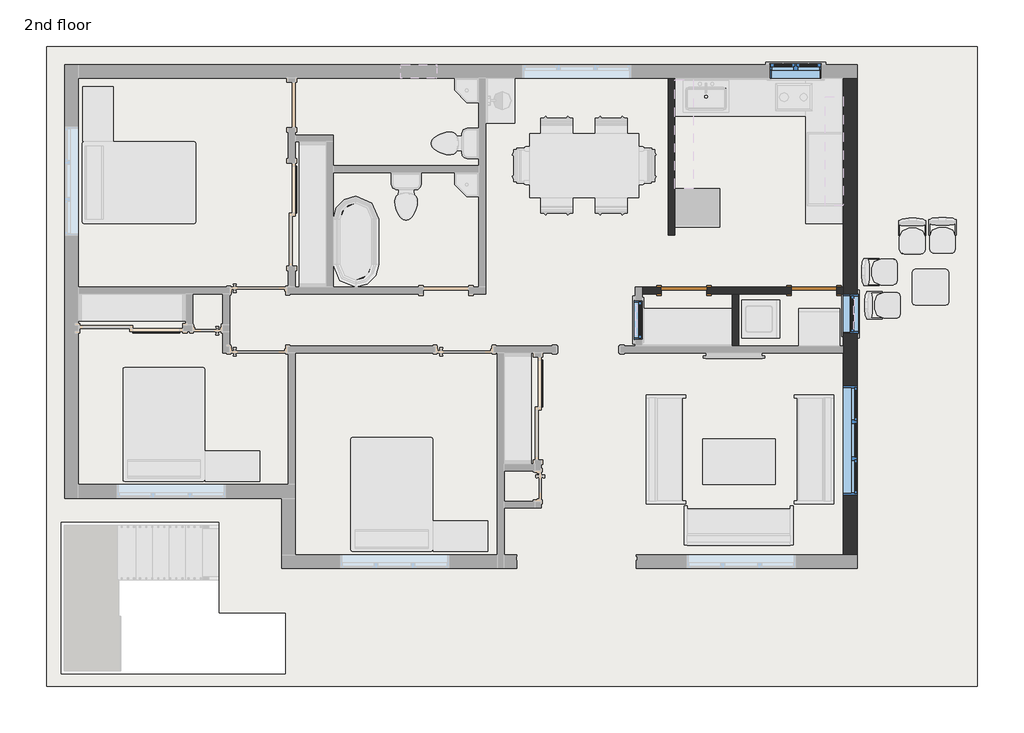
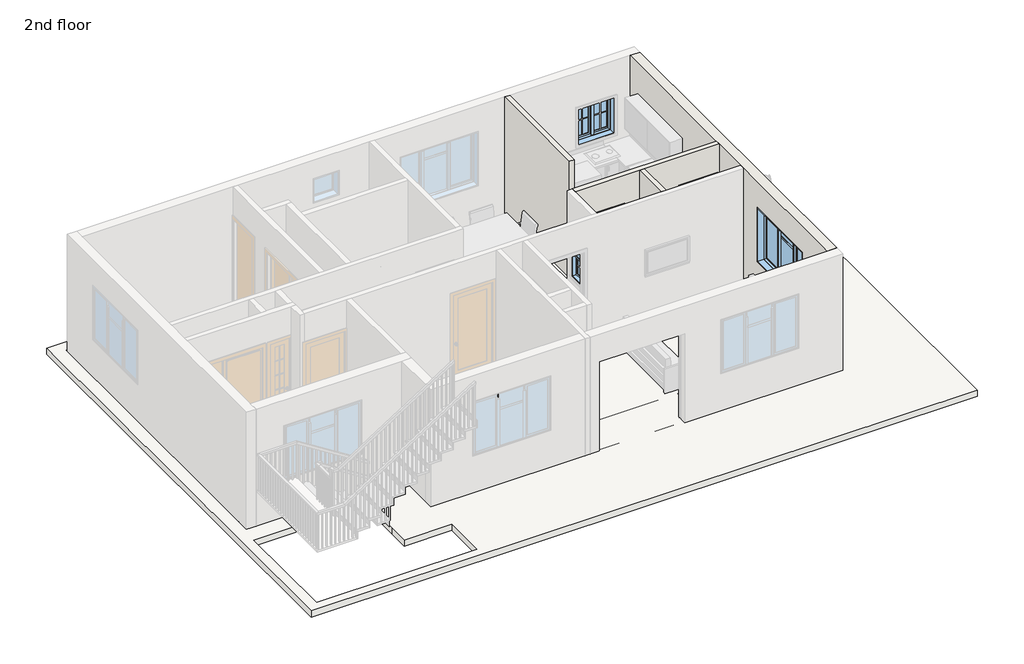
# One storey, part 2 of 4: 18 beams, 4 walls, 4 windows, 2 doors, 1 slab.
"""IFC4 building model written with IfcOpenShell, lengths in millimetres."""

from ifc_helpers import new_model, si_unit, frame, origin, place, context, project, spatial, polyline, outline, extrude, faceted_brep, transform, mapped, element, save
from components import door_214872d5, window_339605e1, window_7a1f68bc, window_251dd907, window_d2058a86

model = new_model("IFC4")

# Units and contexts
model_context = context("Model", 3, world=origin())
ifc_project = project(units=[si_unit("LENGTHUNIT", "METRE", prefix="MILLI")], contexts=[model_context])

# Site, building, storey
site = spatial("IfcSite", under=ifc_project)
building = spatial("IfcBuilding", under=site)
storey = spatial("IfcBuildingStorey", under=building, Name="2nd floor", Elevation=7010.4)

# Beams
placement = place(None, origin())
element("IfcBeam", 1, ObjectType="Concrete-Rectangular Beam", at=placement, inside=storey, context=model_context, shape_type="Brep", body=[
    faceted_brep([(-8931.9263529, 6644.5661978, 7010.4), (-8931.9263529, 6415.9661978, 7010.4), (-5521.9763529, 6415.9661978, 7010.4), (-5293.3763529, 6415.9661978, 7010.4), (-2264.4263529, 6415.9661978, 7010.4), (-2035.8263529, 6415.9661978, 7010.4), (897.8736471, 6415.9661978, 7010.4), (1126.4736471, 6415.9661978, 7010.4), (3901.4236471, 6415.9661978, 7010.4), (3901.4236471, 6644.5661978, 7010.4), (1164.5736471, 6644.5661978, 7010.4), (1164.5736471, 6454.0661978, 7010.4), (859.7736471, 6454.0661978, 7010.4), (859.7736471, 6644.5661978, 7010.4), (-1997.7263529, 6644.5661978, 7010.4), (-1997.7263529, 6454.0661978, 7010.4), (-2302.5263529, 6454.0661978, 7010.4), (-2302.5263529, 6644.5661978, 7010.4), (-5198.1263529, 6644.5661978, 7010.4), (-5198.1263529, 6454.0661978, 7010.4), (-5502.9263529, 6454.0661978, 7010.4), (-5502.9263529, 6644.5661978, 7010.4), (-8931.9263529, 6415.9661978, 6705.6), (-5521.9763529, 6415.9661978, 6705.6), (-5293.3763529, 6415.9661978, 6705.6), (-2264.4263529, 6415.9661978, 6705.6), (-2035.8263529, 6415.9661978, 6705.6), (897.8736471, 6415.9661978, 6705.6), (1126.4736471, 6415.9661978, 6705.6), (3901.4236471, 6415.9661978, 6705.6), (-8931.9263529, 6644.5661978, 6705.6), (-5502.9263529, 6644.5661978, 6705.6), (-5502.9263529, 6454.0661978, 6705.6), (-5198.1263529, 6454.0661978, 6705.6), (-5198.1263529, 6644.5661978, 6705.6), (-2302.5263529, 6644.5661978, 6705.6), (-2302.5263529, 6454.0661978, 6705.6), (-1997.7263529, 6454.0661978, 6705.6), (-1997.7263529, 6644.5661978, 6705.6), (859.7736471, 6644.5661978, 6705.6), (859.7736471, 6454.0661978, 6705.6), (1164.5736471, 6454.0661978, 6705.6), (1164.5736471, 6644.5661978, 6705.6), (3901.4236471, 6644.5661978, 6705.6)], [[[0, 1, 2, 3, 4, 5, 6, 7, 8, 9, 10, 11, 12, 13, 14, 15, 16, 17, 18, 19, 20, 21]], [[1, 22, 23, 24, 25, 26, 27, 28, 29, 8, 7, 6, 5, 4, 3, 2]], [[22, 30, 31, 32, 33, 34, 35, 36, 37, 38, 39, 40, 41, 42, 43, 29, 28, 27, 26, 25, 24, 23]], [[9, 43, 42, 10]], [[1, 0, 30, 22]], [[9, 8, 29, 43]], [[33, 19, 18, 34]], [[19, 33, 32, 20]], [[20, 32, 31, 21]], [[30, 0, 21, 31]], [[37, 15, 14, 38]], [[15, 37, 36, 16]], [[16, 36, 35, 17]], [[34, 18, 17, 35]], [[41, 11, 10, 42]], [[11, 41, 40, 12]], [[12, 40, 39, 13]], [[38, 14, 13, 39]]]),
])
element("IfcBeam", 2, ObjectType="Concrete-Rectangular Beam", at=placement, inside=storey, context=model_context, shape_type="Brep", body=[
    faceted_brep([(3901.4236471, -1470.7338022, 7010.4), (4130.0236471, -1470.7338022, 7010.4), (4130.0236471, 1748.7161978, 7010.4), (3901.4236471, 1748.7161978, 7010.4), (3901.4236471, 1729.6661978, 7010.4), (3901.4236471, 34.2161978, 7010.4), (3901.4236471, -194.3838022, 7010.4), (3901.4236471, -588.0838022, 7010.4), (3901.4236471, -816.6838022, 7010.4), (3901.4236471, -1470.7338022, 6705.6), (3901.4236471, 1748.7161978, 6705.6), (3901.4236471, 1729.6661978, 6705.6), (3901.4236471, 34.2161978, 6705.6), (3901.4236471, -194.3838022, 6705.6), (3901.4236471, -588.0838022, 6705.6), (3901.4236471, -816.6838022, 6705.6), (4130.0236471, -1470.7338022, 6705.6), (4130.0236471, 1748.7161978, 6705.6)], [[[0, 1, 2, 3, 4, 5, 6, 7, 8]], [[9, 0, 8, 7, 6, 5, 4, 3, 10, 11, 12, 13, 14, 15]], [[16, 9, 15, 14, 13, 12, 11, 10, 17]], [[1, 16, 17, 2]], [[1, 0, 9, 16]], [[3, 2, 17, 10]]]),
    faceted_brep([(3901.4236471, 6377.8661978, 7010.4), (4130.0236471, 6377.8661978, 7010.4), (4130.0236471, 6377.8661978, 6705.6), (3901.4236471, 6377.8661978, 6705.6), (4130.0236471, 2053.5161978, 7010.4), (3901.4236471, 2053.5161978, 7010.4), (3901.4236471, 2053.5161978, 6705.6), (4130.0236471, 2053.5161978, 6705.6), (3901.4236471, 5558.7161978, 7010.4), (3901.4236471, 5330.1161978, 7010.4), (3901.4236471, 5044.3661978, 7010.4), (3901.4236471, 4815.7661978, 7010.4), (3901.4236471, 3012.3661978, 7010.4), (3901.4236471, 2783.7661978, 7010.4), (3901.4236471, 5558.7161978, 6705.6), (3901.4236471, 5330.1161978, 6705.6), (3901.4236471, 5044.3661978, 6705.6), (3901.4236471, 4815.7661978, 6705.6), (3901.4236471, 3012.3661978, 6705.6), (3901.4236471, 2783.7661978, 6705.6)], [[[0, 1, 2, 3]], [[4, 5, 6, 7]], [[1, 0, 8, 9, 10, 11, 12, 13, 5, 4]], [[0, 3, 14, 15, 16, 17, 18, 19, 6, 5, 13, 12, 11, 10, 9, 8]], [[3, 2, 7, 6, 19, 18, 17, 16, 15, 14]], [[2, 1, 4, 7]]]),
])
element("IfcBeam", 3, ObjectType="Concrete-Rectangular Beam", at=placement, inside=storey, context=model_context, shape_type="Brep", body=[
    faceted_brep([(3901.4236471, -1737.4338022, 7010.4), (3901.4236471, -1508.8338022, 7010.4), (-1731.0263529, -1508.8338022, 7010.4), (-1959.6263529, -1508.8338022, 7010.4), (-5293.3763529, -1508.8338022, 7010.4), (-5293.3763529, -1737.4338022, 7010.4), (-1997.7263529, -1737.4338022, 7010.4), (-1997.7263529, -1546.9338022, 7010.4), (-1692.9263529, -1546.9338022, 7010.4), (-1692.9263529, -1737.4338022, 7010.4), (859.7736471, -1737.4338022, 7010.4), (859.7736471, -1546.9338022, 7010.4), (1164.5736471, -1546.9338022, 7010.4), (1164.5736471, -1737.4338022, 7010.4), (3901.4236471, -1508.8338022, 6705.6), (-1731.0263529, -1508.8338022, 6705.6), (-1959.6263529, -1508.8338022, 6705.6), (-5293.3763529, -1508.8338022, 6705.6), (3901.4236471, -1737.4338022, 6705.6), (1164.5736471, -1737.4338022, 6705.6), (1164.5736471, -1546.9338022, 6705.6), (859.7736471, -1546.9338022, 6705.6), (859.7736471, -1737.4338022, 6705.6), (-1692.9263529, -1737.4338022, 6705.6), (-1692.9263529, -1546.9338022, 6705.6), (-1997.7263529, -1546.9338022, 6705.6), (-1997.7263529, -1737.4338022, 6705.6), (-5293.3763529, -1737.4338022, 6705.6)], [[[0, 1, 2, 3, 4, 5, 6, 7, 8, 9, 10, 11, 12, 13]], [[1, 14, 15, 16, 17, 4, 3, 2]], [[14, 18, 19, 20, 21, 22, 23, 24, 25, 26, 27, 17, 16, 15]], [[5, 27, 26, 6]], [[1, 0, 18, 14]], [[5, 4, 17, 27]], [[21, 11, 10, 22]], [[11, 21, 20, 12]], [[12, 20, 19, 13]], [[18, 0, 13, 19]], [[25, 7, 6, 26]], [[7, 25, 24, 8]], [[8, 24, 23, 9]], [[22, 10, 9, 23]]]),
])
element("IfcBeam", 4, ObjectType="Concrete-Rectangular Beam", at=placement, inside=storey, context=model_context, shape_type="Brep", body=[
    faceted_brep([(-5293.3763529, 6415.9661978, 7010.4), (-5521.9763529, 6415.9661978, 7010.4), (-5521.9763529, 3012.3661978, 7010.4), (-5521.9763529, 2783.7661978, 7010.4), (-5521.9763529, 1958.2661978, 7010.4), (-5521.9763529, 1729.6661978, 7010.4), (-5521.9763529, -327.7338022, 7010.4), (-5521.9763529, -556.3338022, 7010.4), (-5521.9763529, -1470.7338022, 7010.4), (-5293.3763529, -1470.7338022, 7010.4), (-5293.3763529, 1729.6661978, 7010.4), (-5401.3263529, 1729.6661978, 7010.4), (-5401.3263529, 1958.2661978, 7010.4), (-5293.3763529, 1958.2661978, 7010.4), (-5293.3763529, 2783.7661978, 7010.4), (-5293.3763529, 3012.3661978, 7010.4), (-5293.3763529, 5330.1161978, 7010.4), (-5293.3763529, 5558.7161978, 7010.4), (-5293.3763529, 6415.9661978, 6705.6), (-5293.3763529, 1958.2661978, 6705.6), (-5293.3763529, 2783.7661978, 6705.6), (-5293.3763529, 3012.3661978, 6705.6), (-5293.3763529, 5330.1161978, 6705.6), (-5293.3763529, 5558.7161978, 6705.6), (-5521.9763529, 6415.9661978, 6705.6), (-5401.3263529, 1958.2661978, 6705.6), (-5401.3263529, 1729.6661978, 6705.6), (-5293.3763529, 1729.6661978, 6705.6), (-5293.3763529, -1470.7338022, 6705.6), (-5521.9763529, -1470.7338022, 6705.6), (-5521.9763529, -556.3338022, 6705.6), (-5521.9763529, -327.7338022, 6705.6), (-5521.9763529, 1729.6661978, 6705.6), (-5521.9763529, 1958.2661978, 6705.6), (-5521.9763529, 2783.7661978, 6705.6), (-5521.9763529, 3012.3661978, 6705.6)], [[[0, 1, 2, 3, 4, 5, 6, 7, 8, 9, 10, 11, 12, 13, 14, 15, 16, 17]], [[18, 0, 17, 16, 15, 14, 13, 19, 20, 21, 22, 23]], [[24, 18, 23, 22, 21, 20, 19, 25, 26, 27, 28, 29, 30, 31, 32, 33, 34, 35]], [[1, 24, 35, 34, 33, 32, 31, 30, 29, 8, 7, 6, 5, 4, 3, 2]], [[1, 0, 18, 24]], [[9, 8, 29, 28]], [[12, 25, 19, 13]], [[26, 11, 10, 27]], [[11, 26, 25, 12]], [[9, 28, 27, 10]]]),
])
element("IfcBeam", 5, ObjectType="Concrete-Rectangular Beam", at=placement, inside=storey, context=model_context, shape_type="SweptSolid", body=[
    extrude(outline(polyline([(-5521.9763529, -327.7338022), (-5521.9763529, -556.3338022), (-8931.9263529, -556.3338022), (-8931.9263529, -327.7338022), (-5521.9763529, -327.7338022)])), frame((0.0, 0.0, 6705.6), z_axis=(0.0, 0.0, 1.0), x_axis=(1.0, 0.0, 0.0)), (0.0, 0.0, 1.0), 304.8),
])
element("IfcBeam", 6, ObjectType="Concrete-Rectangular Beam", at=placement, inside=storey, context=model_context, shape_type="Brep", body=[
    faceted_brep([(-9160.5263529, 6720.7661978, 7010.4), (-8931.9263529, 6720.7661978, 7010.4), (-8931.9263529, 6720.7661978, 6705.6), (-9160.5263529, 6720.7661978, 6705.6), (-9160.5263529, 6682.6661978, 7010.4), (-8931.9263529, 6682.6661978, 7010.4), (-8931.9263529, 6682.6661978, 6705.6), (-9160.5263529, 6682.6661978, 6705.6)], [[[0, 1, 2, 3]], [[1, 0, 4, 5]], [[2, 1, 5, 6]], [[3, 2, 6, 7]], [[0, 3, 7, 4]], [[5, 4, 7, 6]]]),
    faceted_brep([(-8931.9263529, 6377.8661978, 7010.4), (-9160.5263529, 6377.8661978, 7010.4), (-9160.5263529, 3050.4661978, 7010.4), (-8931.9263529, 3050.4661978, 7010.4), (-8931.9263529, 6377.8661978, 6705.6), (-8931.9263529, 3050.4661978, 6705.6), (-9160.5263529, 6377.8661978, 6705.6), (-9160.5263529, 3050.4661978, 6705.6)], [[[0, 1, 2, 3]], [[4, 0, 3, 5]], [[6, 4, 5, 7]], [[1, 6, 7, 2]], [[1, 0, 4, 6]], [[3, 2, 7, 5]]]),
    faceted_brep([(-8931.9263529, -289.6338022, 7010.4), (-9160.5263529, -289.6338022, 7010.4), (-9160.5263529, -289.6338022, 6705.6), (-8931.9263529, -289.6338022, 6705.6), (-9160.5263529, 2745.6661978, 7010.4), (-8931.9263529, 2745.6661978, 7010.4), (-8931.9263529, 2745.6661978, 6705.6), (-9160.5263529, 2745.6661978, 6705.6), (-8931.9263529, 1729.6661978, 7010.4), (-8931.9263529, 1958.2661978, 7010.4), (-8931.9263529, 1729.6661978, 6705.6), (-8931.9263529, 1958.2661978, 6705.6)], [[[0, 1, 2, 3]], [[4, 5, 6, 7]], [[1, 0, 8, 9, 5, 4]], [[0, 3, 10, 11, 6, 5, 9, 8]], [[3, 2, 7, 6, 11, 10]], [[2, 1, 4, 7]]]),
])
element("IfcBeam", 7, ObjectType="Concrete-Rectangular Beam", at=placement, inside=storey, context=model_context, shape_type="Brep", body=[
    faceted_brep([(-8931.9263529, 3012.3661978, 7010.4), (-8931.9263529, 2783.7661978, 7010.4), (-5521.9763529, 2783.7661978, 7010.4), (-5521.9763529, 3012.3661978, 7010.4), (-8931.9263529, 2783.7661978, 6705.6), (-5521.9763529, 2783.7661978, 6705.6), (-8931.9263529, 3012.3661978, 6705.6), (-5521.9763529, 3012.3661978, 6705.6)], [[[0, 1, 2, 3]], [[1, 4, 5, 2]], [[4, 6, 7, 5]], [[6, 0, 3, 7]], [[1, 0, 6, 4]], [[3, 2, 5, 7]]]),
    faceted_brep([(3901.4236471, 3012.3661978, 7010.4), (3901.4236471, 2783.7661978, 7010.4), (3901.4236471, 2783.7661978, 6705.6), (3901.4236471, 3012.3661978, 6705.6), (-5293.3763529, 2783.7661978, 7010.4), (-5293.3763529, 3012.3661978, 7010.4), (-5293.3763529, 3012.3661978, 6705.6), (-5293.3763529, 2783.7661978, 6705.6), (1126.4736471, 3012.3661978, 7010.4), (897.8736471, 3012.3661978, 7010.4), (-2035.8263529, 3012.3661978, 7010.4), (-2264.4263529, 3012.3661978, 7010.4), (-4601.2263529, 3012.3661978, 7010.4), (-4829.8263529, 3012.3661978, 7010.4), (351.7736471, 2783.7661978, 7010.4), (580.3736471, 2783.7661978, 7010.4), (1977.3736471, 2783.7661978, 7010.4), (2205.9736471, 2783.7661978, 7010.4), (351.7736471, 2783.7661978, 6705.6), (580.3736471, 2783.7661978, 6705.6), (1977.3736471, 2783.7661978, 6705.6), (2205.9736471, 2783.7661978, 6705.6), (-4829.8263529, 3012.3661978, 6705.6), (-4601.2263529, 3012.3661978, 6705.6), (-2264.4263529, 3012.3661978, 6705.6), (-2035.8263529, 3012.3661978, 6705.6), (897.8736471, 3012.3661978, 6705.6), (1126.4736471, 3012.3661978, 6705.6)], [[[0, 1, 2, 3]], [[4, 5, 6, 7]], [[1, 0, 8, 9, 10, 11, 12, 13, 5, 4, 14, 15, 16, 17]], [[2, 1, 17, 16, 15, 14, 4, 7, 18, 19, 20, 21]], [[3, 2, 21, 20, 19, 18, 7, 6, 22, 23, 24, 25, 26, 27]], [[0, 3, 27, 26, 25, 24, 23, 22, 6, 5, 13, 12, 11, 10, 9, 8]]]),
])
element("IfcBeam", 8, ObjectType="Concrete-Rectangular Beam", at=placement, inside=storey, context=model_context, shape_type="Brep", body=[
    faceted_brep([(-8931.9263529, 1958.2661978, 7010.4), (-8931.9263529, 1729.6661978, 7010.4), (-5521.9763529, 1729.6661978, 7010.4), (-5521.9763529, 1958.2661978, 7010.4), (-8931.9263529, 1729.6661978, 6705.6), (-5521.9763529, 1729.6661978, 6705.6), (-8931.9263529, 1958.2661978, 6705.6), (-5521.9763529, 1958.2661978, 6705.6)], [[[0, 1, 2, 3]], [[1, 4, 5, 2]], [[4, 6, 7, 5]], [[6, 0, 3, 7]], [[1, 0, 6, 4]], [[3, 2, 5, 7]]]),
    faceted_brep([(3901.4236471, 1958.2661978, 7010.4), (3901.4236471, 1748.7161978, 7010.4), (3901.4236471, 1729.6661978, 7010.4), (3901.4236471, 1729.6661978, 6705.6), (3901.4236471, 1748.7161978, 6705.6), (3901.4236471, 1958.2661978, 6705.6), (618.4736471, 1729.6661978, 7010.4), (618.4736471, 1958.2661978, 7010.4), (618.4736471, 1958.2661978, 6705.6), (618.4736471, 1729.6661978, 6705.6), (2205.9736471, 1958.2661978, 7010.4), (1977.3736471, 1958.2661978, 7010.4), (1977.3736471, 1958.2661978, 6705.6), (2205.9736471, 1958.2661978, 6705.6)], [[[0, 1, 2, 3, 4, 5]], [[6, 7, 8, 9]], [[2, 1, 0, 10, 11, 7, 6]], [[3, 2, 6, 9]], [[5, 4, 3, 9, 8, 12, 13]], [[0, 5, 13, 12, 8, 7, 11, 10]]]),
    faceted_brep([(-5096.5263529, 1958.2661978, 7010.4), (-5096.5263529, 1729.6661978, 7010.4), (-1959.6263529, 1729.6661978, 7010.4), (-1731.0263529, 1729.6661978, 7010.4), (313.6736471, 1729.6661978, 7010.4), (313.6736471, 1958.2661978, 7010.4), (-5096.5263529, 1729.6661978, 6705.6), (-1959.6263529, 1729.6661978, 6705.6), (-1731.0263529, 1729.6661978, 6705.6), (313.6736471, 1729.6661978, 6705.6), (-5096.5263529, 1958.2661978, 6705.6), (313.6736471, 1958.2661978, 6705.6)], [[[0, 1, 2, 3, 4, 5]], [[1, 6, 7, 8, 9, 4, 3, 2]], [[6, 10, 11, 9, 8, 7]], [[10, 0, 5, 11]], [[1, 0, 10, 6]], [[5, 4, 9, 11]]]),
])
element("IfcBeam", 9, ObjectType="Concrete-Rectangular Beam", at=placement, inside=storey, context=model_context, shape_type="Brep", body=[
    faceted_brep([(-1959.6263529, -1508.8338022, 7010.4), (-1731.0263529, -1508.8338022, 7010.4), (-1731.0263529, -816.6838022, 7010.4), (-1731.0263529, -588.0838022, 7010.4), (-1731.0263529, -194.3838022, 7010.4), (-1731.0263529, 34.2161978, 7010.4), (-1731.0263529, 1729.6661978, 7010.4), (-1959.6263529, 1729.6661978, 7010.4), (-1959.6263529, -1508.8338022, 6705.6), (-1959.6263529, 1729.6661978, 6705.6), (-1731.0263529, -1508.8338022, 6705.6), (-1731.0263529, 1729.6661978, 6705.6), (-1731.0263529, 34.2161978, 6705.6), (-1731.0263529, -194.3838022, 6705.6), (-1731.0263529, -588.0838022, 6705.6), (-1731.0263529, -816.6838022, 6705.6)], [[[0, 1, 2, 3, 4, 5, 6, 7]], [[8, 0, 7, 9]], [[10, 8, 9, 11, 12, 13, 14, 15]], [[1, 10, 15, 14, 13, 12, 11, 6, 5, 4, 3, 2]], [[1, 0, 8, 10]], [[7, 6, 11, 9]]]),
])
element("IfcBeam", 10, ObjectType="Concrete-Rectangular Beam", at=placement, inside=storey, context=model_context, shape_type="SweptSolid", body=[
    extrude(outline(polyline([(3901.4236471, -588.0838022), (3901.4236471, -816.6838022), (-1731.0263529, -816.6838022), (-1731.0263529, -588.0838022), (3901.4236471, -588.0838022)])), frame((0.0, 0.0, 6705.6), z_axis=(0.0, 0.0, 1.0), x_axis=(1.0, 0.0, 0.0)), (0.0, 0.0, 1.0), 304.8),
])
element("IfcBeam", 11, ObjectType="Concrete-Rectangular Beam", at=placement, inside=storey, context=model_context, shape_type="SweptSolid", body=[
    extrude(outline(polyline([(3901.4236471, 34.2161978), (3901.4236471, -194.3838022), (-1731.0263529, -194.3838022), (-1731.0263529, 34.2161978), (3901.4236471, 34.2161978)])), frame((0.0, 0.0, 6705.6), z_axis=(0.0, 0.0, 1.0), x_axis=(1.0, 0.0, 0.0)), (0.0, 0.0, 1.0), 304.8),
])
element("IfcBeam", 12, ObjectType="Concrete-Rectangular Beam", at=placement, inside=storey, context=model_context, shape_type="Brep", body=[
    faceted_brep([(3901.4236471, 5330.1161978, 7010.4), (3901.4236471, 5558.7161978, 7010.4), (1126.4736471, 5558.7161978, 7010.4), (897.8736471, 5558.7161978, 7010.4), (-2035.8263529, 5558.7161978, 7010.4), (-2264.4263529, 5558.7161978, 7010.4), (-5293.3763529, 5558.7161978, 7010.4), (-5293.3763529, 5330.1161978, 7010.4), (-4829.8263529, 5330.1161978, 7010.4), (-4601.2263529, 5330.1161978, 7010.4), (-2264.4263529, 5330.1161978, 7010.4), (-2035.8263529, 5330.1161978, 7010.4), (897.8736471, 5330.1161978, 7010.4), (1126.4736471, 5330.1161978, 7010.4), (3901.4236471, 5330.1161978, 6705.6), (-5293.3763529, 5330.1161978, 6705.6), (-4829.8263529, 5330.1161978, 6705.6), (-4601.2263529, 5330.1161978, 6705.6), (-2264.4263529, 5330.1161978, 6705.6), (-2035.8263529, 5330.1161978, 6705.6), (897.8736471, 5330.1161978, 6705.6), (1126.4736471, 5330.1161978, 6705.6), (3901.4236471, 5558.7161978, 6705.6), (-5293.3763529, 5558.7161978, 6705.6), (-2264.4263529, 5558.7161978, 6705.6), (-2035.8263529, 5558.7161978, 6705.6), (897.8736471, 5558.7161978, 6705.6), (1126.4736471, 5558.7161978, 6705.6)], [[[0, 1, 2, 3, 4, 5, 6, 7, 8, 9, 10, 11, 12, 13]], [[14, 0, 13, 12, 11, 10, 9, 8, 7, 15, 16, 17, 18, 19, 20, 21]], [[22, 14, 21, 20, 19, 18, 17, 16, 15, 23, 24, 25, 26, 27]], [[1, 22, 27, 26, 25, 24, 23, 6, 5, 4, 3, 2]], [[1, 0, 14, 22]], [[7, 6, 23, 15]]]),
])
element("IfcBeam", 13, ObjectType="Concrete-Rectangular Beam", at=placement, inside=storey, context=model_context, shape_type="Brep", body=[
    faceted_brep([(3901.4236471, 4815.7661978, 7010.4), (3901.4236471, 5044.3661978, 7010.4), (1126.4736471, 5044.3661978, 7010.4), (897.8736471, 5044.3661978, 7010.4), (-2035.8263529, 5044.3661978, 7010.4), (-2264.4263529, 5044.3661978, 7010.4), (-4601.2263529, 5044.3661978, 7010.4), (-4601.2263529, 4815.7661978, 7010.4), (-2264.4263529, 4815.7661978, 7010.4), (-2035.8263529, 4815.7661978, 7010.4), (897.8736471, 4815.7661978, 7010.4), (1126.4736471, 4815.7661978, 7010.4), (3901.4236471, 4815.7661978, 6705.6), (-4601.2263529, 4815.7661978, 6705.6), (-2264.4263529, 4815.7661978, 6705.6), (-2035.8263529, 4815.7661978, 6705.6), (897.8736471, 4815.7661978, 6705.6), (1126.4736471, 4815.7661978, 6705.6), (3901.4236471, 5044.3661978, 6705.6), (-4601.2263529, 5044.3661978, 6705.6), (-2264.4263529, 5044.3661978, 6705.6), (-2035.8263529, 5044.3661978, 6705.6), (897.8736471, 5044.3661978, 6705.6), (1126.4736471, 5044.3661978, 6705.6)], [[[0, 1, 2, 3, 4, 5, 6, 7, 8, 9, 10, 11]], [[12, 0, 11, 10, 9, 8, 7, 13, 14, 15, 16, 17]], [[18, 12, 17, 16, 15, 14, 13, 19, 20, 21, 22, 23]], [[1, 18, 23, 22, 21, 20, 19, 6, 5, 4, 3, 2]], [[1, 0, 12, 18]], [[7, 6, 19, 13]]]),
])
element("IfcBeam", 14, ObjectType="Concrete-Rectangular Beam", at=placement, inside=storey, context=model_context, shape_type="Brep", body=[
    faceted_brep([(-4829.8263529, 3012.3661978, 7010.4), (-4601.2263529, 3012.3661978, 7010.4), (-4601.2263529, 4815.7661978, 7010.4), (-4601.2263529, 5044.3661978, 7010.4), (-4601.2263529, 5330.1161978, 7010.4), (-4829.8263529, 5330.1161978, 7010.4), (-4829.8263529, 3012.3661978, 6705.6), (-4829.8263529, 5330.1161978, 6705.6), (-4601.2263529, 3012.3661978, 6705.6), (-4601.2263529, 5330.1161978, 6705.6), (-4601.2263529, 5044.3661978, 6705.6), (-4601.2263529, 4815.7661978, 6705.6)], [[[0, 1, 2, 3, 4, 5]], [[6, 0, 5, 7]], [[8, 6, 7, 9, 10, 11]], [[1, 8, 11, 10, 9, 4, 3, 2]], [[1, 0, 6, 8]], [[5, 4, 9, 7]]]),
])
element("IfcBeam", 15, ObjectType="Concrete-Rectangular Beam", at=placement, inside=storey, context=model_context, shape_type="SweptSolid", body=[
    extrude(outline(polyline([(-2035.8263529, 3012.3661978), (-2264.4263529, 3012.3661978), (-2264.4263529, 4815.7661978), (-2035.8263529, 4815.7661978), (-2035.8263529, 3012.3661978)])), frame((0.0, 0.0, 6705.6), z_axis=(0.0, 0.0, 1.0), x_axis=(1.0, 0.0, 0.0)), (0.0, 0.0, 1.0), 304.8),
    extrude(outline(polyline([(-2264.4263529, 6415.9661978), (-2035.8263529, 6415.9661978), (-2035.8263529, 5558.7161978), (-2264.4263529, 5558.7161978), (-2264.4263529, 6415.9661978)])), frame((0.0, 0.0, 6705.6), z_axis=(0.0, 0.0, 1.0), x_axis=(1.0, 0.0, 0.0)), (0.0, 0.0, 1.0), 304.8),
    extrude(outline(polyline([(-2264.4263529, 5330.1161978), (-2035.8263529, 5330.1161978), (-2035.8263529, 5044.3661978), (-2264.4263529, 5044.3661978), (-2264.4263529, 5330.1161978)])), frame((0.0, 0.0, 6705.6), z_axis=(0.0, 0.0, 1.0), x_axis=(1.0, 0.0, 0.0)), (0.0, 0.0, 1.0), 304.8),
])
element("IfcBeam", 16, ObjectType="Concrete-Rectangular Beam", at=placement, inside=storey, context=model_context, shape_type="SweptSolid", body=[
    extrude(outline(polyline([(1126.4736471, 3012.3661978), (897.8736471, 3012.3661978), (897.8736471, 4815.7661978), (1126.4736471, 4815.7661978), (1126.4736471, 3012.3661978)])), frame((0.0, 0.0, 6705.6), z_axis=(0.0, 0.0, 1.0), x_axis=(1.0, 0.0, 0.0)), (0.0, 0.0, 1.0), 304.8),
    extrude(outline(polyline([(897.8736471, 6415.9661978), (1126.4736471, 6415.9661978), (1126.4736471, 5558.7161978), (897.8736471, 5558.7161978), (897.8736471, 6415.9661978)])), frame((0.0, 0.0, 6705.6), z_axis=(0.0, 0.0, 1.0), x_axis=(1.0, 0.0, 0.0)), (0.0, 0.0, 1.0), 304.8),
    extrude(outline(polyline([(897.8736471, 5330.1161978), (1126.4736471, 5330.1161978), (1126.4736471, 5044.3661978), (897.8736471, 5044.3661978), (897.8736471, 5330.1161978)])), frame((0.0, 0.0, 6705.6), z_axis=(0.0, 0.0, 1.0), x_axis=(1.0, 0.0, 0.0)), (0.0, 0.0, 1.0), 304.8),
])
element("IfcBeam", 17, ObjectType="Concrete-Rectangular Beam", at=placement, inside=storey, context=model_context, shape_type="SweptSolid", body=[
    extrude(outline(polyline([(351.7736471, 2783.7661978), (580.3736471, 2783.7661978), (580.3736471, 1958.2661978), (351.7736471, 1958.2661978), (351.7736471, 2783.7661978)])), frame((0.0, 0.0, 6705.6), z_axis=(0.0, 0.0, 1.0), x_axis=(1.0, 0.0, 0.0)), (0.0, 0.0, 1.0), 304.8),
])
element("IfcBeam", 18, ObjectType="Concrete-Rectangular Beam", at=placement, inside=storey, context=model_context, shape_type="SweptSolid", body=[
    extrude(outline(polyline([(1977.3736471, 2783.7661978), (2205.9736471, 2783.7661978), (2205.9736471, 1958.2661978), (1977.3736471, 1958.2661978), (1977.3736471, 2783.7661978)])), frame((0.0, 0.0, 6705.6), z_axis=(0.0, 0.0, 1.0), x_axis=(1.0, 0.0, 0.0)), (0.0, 0.0, 1.0), 304.8),
])

# Doors
door_shape = door_214872d5(model_context)
element("IfcDoor", 19, ObjectType="Single-Flush : 30\" x 84\"", at=placement, inside=storey, context=model_context, shape_type="MappedRepresentation", body=[
    mapped(door_shape, transform((3406.1236471, 2891.7161978, 7010.4), x_axis=(1.0, 0.0, 0.0), y_axis=(0.0, 1.0, 0.0), z_axis=(0.0, 0.0, 1.0))),
])
element("IfcDoor", 20, ObjectType="Single-Flush : 30\" x 84\"", at=placement, inside=storey, context=model_context, shape_type="MappedRepresentation", body=[
    mapped(door_shape, transform((1228.0736471, 2891.7161978, 7010.4), x_axis=(1.0, 0.0, 0.0), y_axis=(0.0, 1.0, 0.0), z_axis=(0.0, 0.0, 1.0))),
])

# Slab
element("IfcSlab", 21, ObjectType="Generic - 6\"", at=placement, inside=storey, context=model_context, shape_type="SweptSolid", body=[
    extrude(outline(polyline([(6149.3236471, 6987.4661978), (6149.3236471, -3750.3838022), (-9465.3263529, -3750.3838022), (-9465.3263529, 6987.4661978), (6149.3236471, 6987.4661978)]), holes=[polyline([(-6576.0763529, -1000.8338022), (-9217.6763529, -1000.8338022), (-9217.6763529, -3540.8338022), (-5458.4763529, -3540.8338022), (-5458.4763529, -2524.8338022), (-6576.0763529, -2524.8338022), (-6576.0763529, -2016.8338022), (-6576.0763529, -1000.8338022)])]), frame((0.0, 0.0, 6858.0), z_axis=(0.0, 0.0, 1.0), x_axis=(1.0, 0.0, 0.0)), (0.0, 0.0, 1.0), 152.4),
])

# Walls
element("IfcWall", 22, ObjectType="Generic - 4.5\"", at=placement, inside=storey, context=model_context, shape_type="SweptSolid", body=[
    extrude(outline(polyline([(1075.6736471, 6454.0661978), (1075.6736471, 3825.1661978), (961.3736471, 3825.1661978), (961.3736471, 6454.0661978), (1075.6736471, 6454.0661978)])), frame((0.0, 0.0, 7010.4), z_axis=(0.0, 0.0, 1.0), x_axis=(1.0, 0.0, 0.0)), (0.0, 0.0, 1.0), 2895.6),
])
element("IfcWall", 23, ObjectType="Generic - 4.5\"", at=placement, inside=storey, context=model_context, shape_type="Brep", body=[
    faceted_brep([(1609.0736471, 2834.5661978, 9144.0), (1609.0736471, 2834.5661978, 7010.4), (2034.5236471, 2834.5661978, 7010.4), (2148.8236471, 2834.5661978, 7010.4), (3025.1236471, 2834.5661978, 7010.4), (3025.1236471, 2834.5661978, 9144.0), (3787.1236471, 2834.5661978, 9144.0), (3787.1236471, 2834.5661978, 7010.4), (3901.4236471, 2834.5661978, 7010.4), (3901.4236471, 2834.5661978, 9906.0), (2148.8236471, 2834.5661978, 9906.0), (2034.5236471, 2834.5661978, 9906.0), (523.2236471, 2834.5661978, 9906.0), (523.2236471, 2834.5661978, 7010.4), (847.0736471, 2834.5661978, 7010.4), (847.0736471, 2834.5661978, 9144.0), (3025.1236471, 2948.8661978, 7010.4), (1609.0736471, 2948.8661978, 7010.4), (1609.0736471, 2948.8661978, 9144.0), (847.0736471, 2948.8661978, 9144.0), (847.0736471, 2948.8661978, 7010.4), (523.2236471, 2948.8661978, 7010.4), (523.2236471, 2948.8661978, 9906.0), (3901.4236471, 2948.8661978, 9906.0), (3901.4236471, 2948.8661978, 7010.4), (3787.1236471, 2948.8661978, 7010.4), (3787.1236471, 2948.8661978, 9144.0), (3025.1236471, 2948.8661978, 9144.0)], [[[0, 1, 2, 3, 4, 5, 6, 7, 8, 9, 10, 11, 12, 13, 14, 15]], [[16, 17, 18, 19, 20, 21, 22, 23, 24, 25, 26, 27]], [[8, 7, 25, 24]], [[14, 13, 21, 20]], [[4, 3, 2, 1, 17, 16]], [[12, 11, 10, 9, 23, 22]], [[13, 12, 22, 21]], [[9, 8, 24, 23]], [[26, 25, 7, 6]], [[27, 26, 6, 5]], [[16, 27, 5, 4]], [[18, 17, 1, 0]], [[19, 18, 0, 15]], [[20, 19, 15, 14]]]),
])
element("IfcWall", 24, ObjectType="Generic - 4.5\"", at=placement, inside=storey, context=model_context, shape_type="SweptSolid", body=[
    extrude(outline(polyline([(2148.8236471, 2834.5661978), (2148.8236471, 1958.2661978), (2034.5236471, 1958.2661978), (2034.5236471, 2834.5661978), (2148.8236471, 2834.5661978)])), frame((0.0, 0.0, 7010.4), z_axis=(0.0, 0.0, 1.0), x_axis=(1.0, 0.0, 0.0)), (0.0, 0.0, 1.0), 2895.6),
])
element("IfcWall", 25, ObjectType="Generic - 9\"", at=placement, inside=storey, context=model_context, shape_type="Brep", body=[
    faceted_brep([(4130.0236471, -1546.9338022, 7010.4), (4130.0236471, 6454.0661978, 7010.4), (4130.0236471, 6454.0661978, 9906.0), (4130.0236471, -1546.9338022, 9906.0), (4130.0236471, 2828.2161978, 8991.6), (4130.0236471, 2828.2161978, 7924.8), (4130.0236471, 2167.8161978, 7924.8), (4130.0236471, 2167.8161978, 8991.6), (4130.0236471, -537.2838022, 9271.0), (4130.0236471, 1291.5161978, 9271.0), (4130.0236471, 1291.5161978, 7924.8), (4130.0236471, -537.2838022, 7924.8), (3901.4236471, -1546.9338022, 7010.4), (3901.4236471, -1546.9338022, 9906.0), (3901.4236471, 1843.9661978, 9906.0), (3901.4236471, 1958.2661978, 9906.0), (3901.4236471, 2834.5661978, 9906.0), (3901.4236471, 2948.8661978, 9906.0), (3901.4236471, 6454.0661978, 9906.0), (3901.4236471, 6454.0661978, 7010.4), (3901.4236471, 2948.8661978, 7010.4), (3901.4236471, 2834.5661978, 7010.4), (3901.4236471, 1958.2661978, 7010.4), (3901.4236471, 1843.9661978, 7010.4), (3901.4236471, 2828.2161978, 8991.6), (3901.4236471, 2167.8161978, 8991.6), (3901.4236471, 2167.8161978, 7924.8), (3901.4236471, 2828.2161978, 7924.8), (3901.4236471, -537.2838022, 9271.0), (3901.4236471, -537.2838022, 7924.8), (3901.4236471, 1291.5161978, 7924.8), (3901.4236471, 1291.5161978, 9271.0)], [[[0, 1, 2, 3], [4, 5, 6, 7], [8, 9, 10, 11]], [[12, 13, 14, 15, 16, 17, 18, 19, 20, 21, 22, 23], [24, 25, 26, 27], [28, 29, 30, 31]], [[1, 0, 12, 23, 22, 21, 20, 19]], [[3, 2, 18, 17, 16, 15, 14, 13]], [[0, 3, 13, 12]], [[2, 1, 19, 18]], [[5, 4, 24, 27]], [[6, 5, 27, 26]], [[7, 6, 26, 25]], [[4, 7, 25, 24]], [[29, 28, 8, 11]], [[30, 29, 11, 10]], [[31, 30, 10, 9]], [[28, 31, 9, 8]]]),
])

# Windows
window_shape = window_339605e1(model_context)
element("IfcWindow", 26, ObjectType="Window-Casement-Double : 34\" x 36\"", at=placement, inside=storey, context=model_context, shape_type="MappedRepresentation", body=[
    mapped(window_shape, transform((3101.3236471, 6568.3661978, 7188.2), x_axis=(1.0, 0.0, 0.0), y_axis=(0.0, 1.0, 0.0), z_axis=(0.0, 0.0, 1.0))),
])
window_2_shape = window_7a1f68bc(model_context)
element("IfcWindow", 27, ObjectType="Window-Casement-Triple-Middle-Transom : 72\" x 53\"", at=placement, inside=storey, context=model_context, shape_type="MappedRepresentation", body=[
    mapped(window_2_shape, transform((4015.7236471, 377.1161978, 7010.4), x_axis=(0.0, -1.0, 0.0), y_axis=(1.0, 0.0, 0.0), z_axis=(0.0, 0.0, 1.0))),
])
window_3_shape = window_251dd907(model_context)
element("IfcWindow", 28, ObjectType="Window-Double-Hung : 26\" x 42\"", at=placement, inside=storey, context=model_context, shape_type="MappedRepresentation", body=[
    mapped(window_3_shape, transform((4015.7236471, 2498.0161978, 7010.4), x_axis=(0.0, -1.0, 0.0), y_axis=(1.0, 0.0, 0.0), z_axis=(0.0, 0.0, 1.0))),
])
window_4_shape = window_d2058a86(model_context)
element("IfcWindow", 29, ObjectType="Window-Double-Hung : 26\" x 42\"", at=placement, inside=storey, context=model_context, shape_type="MappedRepresentation", body=[
    mapped(window_4_shape, transform((466.0736471, 2396.4161978, 7010.4), x_axis=(0.0, -1.0, 0.0), y_axis=(1.0, 0.0, 0.0), z_axis=(0.0, 0.0, 1.0))),
])

save(model, "model.ifc")

# Revit data of these elements
# Type "Concrete-Rectangular Beam"
#   Assembly Code = "B10"
#   Length [instance default] = 5' - 0"
#   b = 0' - 9"
#   h = 1' - 0"
#   Structural Material [instance default] = Concrete, Cast-in-Place gray
# Type "Single-Flush : 30\" x 84\""
#   Type Mark = "4"
#   Construction Type Id = "MDOOR"
#   Assembly Code = "C1020"
#   Analytic Construction = "Metal"
#   Thickness = 0' - 2"
#   Heat Transfer Coefficient (U) = 0.651978 BTU/(h·ft²·°F)
#   Height = 7' - 0"
#   Trim Projection Ext = 0' - 1"
#   Trim Projection Int = 0' - 1"
#   Trim Width = 0' - 3"
#   Width = 2' - 6"
#   Define Thermal Properties by = 1
#   Define Thermal Properties by = 1
#   Door Material = Door - Panel
#   Frame Material = Door - Frame
#   Visual Light Transmittance = 0
#   Solar Heat Gain Coefficient = 0
#   Function = (empty or 0)
#   Wall Closure = (empty or 0)
# Type "Generic - 6\""
#   Assembly Code = "B1010"
#   Function = 0
#   Layers, outside or top first: 0' - 6" no material (function 1)
# Type "Generic - 4.5\""
#   Assembly Code = "B2010"
#   Layers, outside or top first: 0' - 4 1/2" no material (function 1)
# Type "Generic - 9\""
#   Assembly Code = "B2010"
#   Layers, outside or top first: 0' - 9" no material (function 1)
# Type "Window-Casement-Double : 34\" x 36\""
#   Type Mark = "14"
#   Fire Rating = "0.5h"
#   Assembly Code = "B2020100"
#   Analytic Construction = "Double glazing - domestic"
#   Frame Extension [instance default] = 0' - 0 1/4"
#   Window Inset [instance default] = 0' - 0"
#   Wall Thickness [instance default] = 0' - 6"
#   Interior Wall Closure [instance default] = 0' - 2 1/4"
#   Half Width = 1' - 5"
#   Visual Light Transmittance = 0.81
#   Thermal Resistance (R) = 1.8146 (h·ft²·°F)/BTU
#   Solar Heat Gain Coefficient = 0.76
#   Rough Width = 2' - 10 1/2"
#   Rough Height = 3' - 0 1/2"
#   Height = 3' - 0"
#   Heat Transfer Coefficient (U) = 0.5511 BTU/(h·ft²·°F)
#   Exterior Wall Closure [instance default] = 0' - 1 1/4"
#   Extension Jamb [instance default] = 0' - 2 1/4"
#   Default Sill Height = 3' - 0"
#   Width = 2' - 10"
#   Define Thermal Properties by = 0
#   Muntin Visibility = yes
#   Interior Trim Visibility [instance default] = yes
#   Exterior Trim Visibility [instance default] = yes
#   Extension Jamb Visibility [instance default] = yes
#   Interior Trim Material = Wood - Stained
#   Muntin Pattern = Muntin Pattern_2x2 : Muntin Pattern_2x2
#   Interior Trim = Trim-Window-Interior-Flat : Picture Frame
#   Interior Frame Material = Wood - Stained
#   Glass Panel Material = Glass
#   Exterior Trim Material = Clad - White
#   Exterior Trim = Trim-Window-Exterior-Flat : with Sill
#   Exterior Frame Material = Clad - White
#   Wall Closure = (empty or 0)
# Type "Window-Casement-Triple-Middle-Transom : 72\" x 53\""
#   Type Mark = "18"
#   Fire Rating = "0.5h"
#   Assembly Code = "B2020100"
#   Analytic Construction = "Double glazing - domestic"
#   Window Width = 2' - 0"
#   Window Inset [instance default] = 0' - 0 5/8"
#   Wall Thickness [instance default] = 0' - 6"
#   Visual Light Transmittance = 0.81
#   Transom Height Ratio = 0.3
#   Thermal Resistance (R) = 1.8146 (h·ft²·°F)/BTU
#   Solar Heat Gain Coefficient = 0.76
#   Rough Width = 6' - 0 1/2"
#   Rough Height = 4' - 5 1/2"
#   Heat Transfer Coefficient (U) = 0.5511 BTU/(h·ft²·°F)
#   Height = 4' - 5"
#   Transom Height = 1' - 3.9"
#   Frame Gap 3 [instance default] = 0' - 1 83/128"
#   Frame Gap 2 [instance default] = 0' - 0 5/8"
#   Frame Gap 1 = 0' - 1 51/128"
#   Default Sill Height = 3' - 0"
#   Width = 6' - 0"
#   Frame Material = Metal - Aluminum
#   Glass Panel Material = Glass
#   Wall Closure = (empty or 0)
# Type "Window-Double-Hung : 26\" x 42\""
#   Type Mark = "11"
#   Fire Rating = "0.5h"
#   Construction Type Id = "DG-DR"
#   Assembly Code = "B2020100"
#   Analytic Construction = "Double glazing - domestic"
#   Wall Thickness [instance default] = 0' - 6"
#   Window Inset [instance default] = 0' - 0"
#   Visual Light Transmittance = 0.81
#   Thermal Resistance (R) = 1.8146 (h·ft²·°F)/BTU
#   Solar Heat Gain Coefficient = 0.76
#   Muntin Width = 1' - 8"
#   Muntin Height = 1' - 5 1/8"
#   Interior Wall Closure [instance default] = 0' - 1 1/2"
#   Rough Width = 2' - 2 1/2"
#   Rough Height = 3' - 6 1/2"
#   Frame Extension [instance default] = 0' - 1 1/4"
#   Exterior Wall Closure [instance default] = 0' - 0 1/2"
#   Extension Jamb [instance default] = 0' - 1 1/2"
#   Heat Transfer Coefficient (U) = 0.5511 BTU/(h·ft²·°F)
#   Height = 3' - 6"
#   Width = 2' - 2"
#   Define Thermal Properties by = 1
#   Top Muntin Visibility = yes
#   Indicator Visibility [instance default] = yes
#   Extension Jamb Visibility [instance default] = yes
#   Interior Trim Visibility [instance default] = yes
#   Exterior Trim Visibility [instance default] = yes
#   Define Thermal Properties by = 1
#   Bottom Muntin Visibility = yes
#   Muntin Pattern = Muntin Pattern_2x2 : Muntin Pattern_2x2
#   Interior Trim Material = Wood - Stained
#   Interior Trim = Trim-Window-Interior-Flat : Picture Frame
#   Exterior Trim Material = Clad - White
#   Exterior Trim = Trim-Window-Exterior-Flat : with Sill
#   Glass Panel Material = Glass
#   Exterior Frame Material = Clad - White
#   Interior Frame Material = Wood - Stained
#   Wall Closure = (empty or 0)
# Elements 1, 2, 3, 4, 5, 6, 7, 8, 9, 10, 11, 12, 13, 14, 15, 16, 17, 18 (IfcBeam, "Concrete-Rectangular Beam")
#   Structural Material = Concrete, Cast-in-Place gray
#   Phase Created = New Construction
#   Materials on its faces: "Concrete, Cast-in-Place gray"
# Elements 19, 20 (IfcDoor, "Single-Flush : 30\" x 84\"")
#   Phase Created = New Construction
#   Materials on its faces: "Door - Frame", "Door - Panel"
# Element 21 (IfcSlab, "Generic - 6\"")
#   Height Offset From Level = 0' - 0"
#   Phase Created = New Construction
#   Materials on its faces: "Default Floor"
# Elements 22, 23, 24 (IfcWall, "Generic - 4.5\"")
#   Top Offset = 0' - 0"
#   Base Offset = 0' - 0"
#   Unconnected Height = 9' - 6"
#   wall height = 9' - 6"
#   Phase Created = New Construction
#   Base Constraint = 2nd floor
#   Materials on its faces: "Default Wall"
# Element 25 (IfcWall, "Generic - 9\"")
#   Top Offset = 0' - 0"
#   Base Offset = 0' - 0"
#   Unconnected Height = 9' - 6"
#   wall height = 9' - 6"
#   Phase Created = New Construction
#   Base Constraint = 2nd floor
#   Materials on its faces: "Default Wall"
# Element 26 (IfcWindow, "Window-Casement-Double : 34\" x 36\"")
#   Mark = "25"
#   Window Inset = 0' - 0"
#   Interior Wall Closure = 0' - 2 1/4"
#   Frame Extension = 0' - 0 1/4"
#   Exterior Wall Closure = 0' - 1 1/4"
#   Interior Trim Visibility = yes
#   Exterior Trim Visibility = yes
#   Phase Created = New Construction
#   Materials on its faces: "Wood - Stained", "Glass", "Clad - White"
# Element 27 (IfcWindow, "Window-Casement-Triple-Middle-Transom : 72\" x 53\"")
#   Mark = "32"
#   Window Inset = 0' - 0 5/8"
#   Frame Gap 3 = 0' - 1 83/128"
#   Frame Gap 2 = 0' - 0 5/8"
#   Phase Created = New Construction
#   Materials on its faces: "Metal - Aluminum", "Glass"
# Element 28 (IfcWindow, "Window-Double-Hung : 26\" x 42\"")
#   Mark = "26"
#   Window Inset = 0' - 0"
#   Interior Wall Closure = 0' - 1 1/2"
#   Frame Extension = 0' - 1 1/4"
#   Exterior Wall Closure = 0' - 0 1/2"
#   Interior Trim Visibility = yes
#   Indicator Visibility = yes
#   Exterior Trim Visibility = yes
#   Phase Created = New Construction
#   Materials on its faces: "Wood - Stained", "Glass", "Clad - White"
# Element 29 (IfcWindow, "Window-Double-Hung : 26\" x 42\"")
#   Mark = "27"
#   Window Inset = 0' - 0"
#   Interior Wall Closure = 0' - 1 1/2"
#   Frame Extension = 0' - 1 1/4"
#   Exterior Wall Closure = 0' - 0 1/2"
#   Interior Trim Visibility = yes
#   Indicator Visibility = yes
#   Exterior Trim Visibility = yes
#   Phase Created = New Construction
#   Materials on its faces: "Wood - Stained", "Glass", "Clad - White"
# Materials
#   "Concrete, Cast-in-Place gray": class "Concrete", colour RGB 192 192 192, transparency 0, Description = "Cast-in-place concrete", Cost = 0
#   "Door - Panel": class "Wood", colour RGB 210 159 95, transparency 0, Cost = 0
#   "Door - Frame": colour RGB 118 70 51, transparency 0, Cost = 0
#   "Wood - Stained": class "Wood", colour RGB 224 178 126, transparency 0, Cost = 0
#   "Glass": class "Glass", colour RGB 0 128 192, transparency 0.75, Description = "Soda Lime Glass", Cost = 0
#   "Clad - White": class "Wood", colour RGB 242 242 238, transparency 0, Cost = 0
#   "Metal - Aluminum": class "Metal", colour RGB 247 247 247, transparency 0
#   "Default Floor": colour RGB 128 128 128, transparency 0, Cost = 0
#   "Default Wall": colour RGB 128 128 128, transparency 0, Cost = 0
